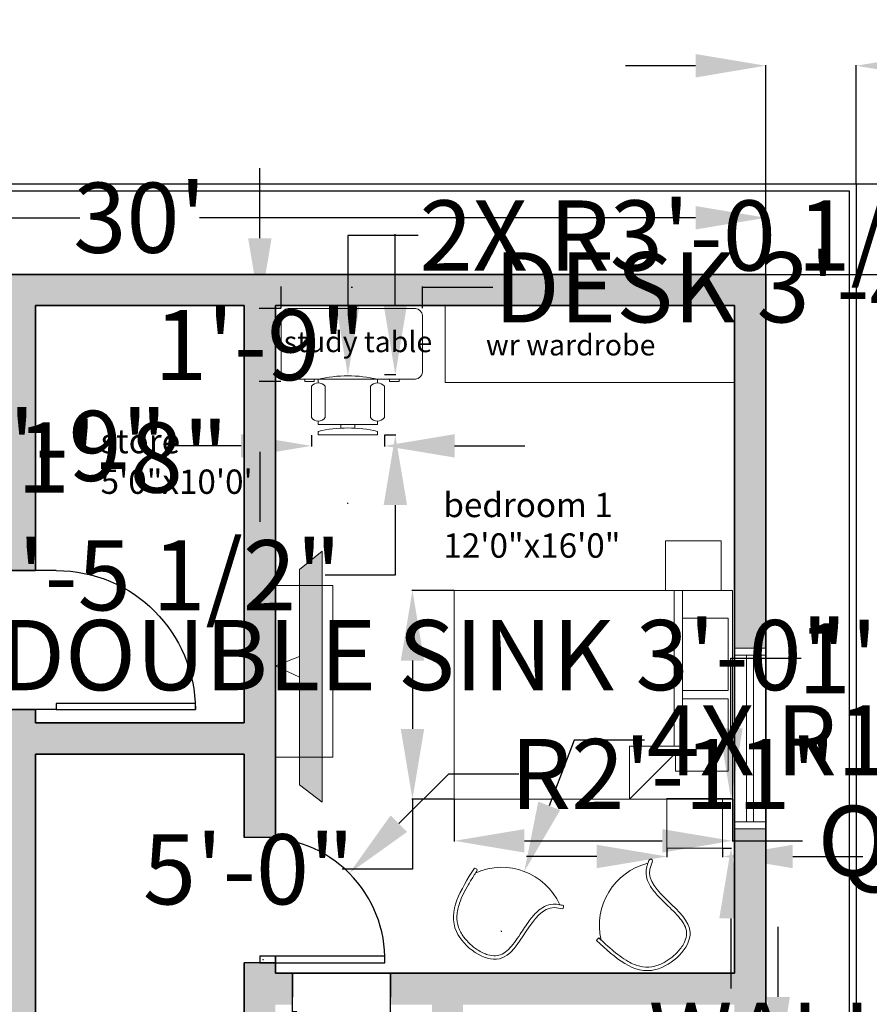
# Model space of a CAD drawing. Units: inches. Extents: x 1202 to 2101, y 998 to 1743.
# Tile 3 of 4: x 1553 to 1798, y 1460 to 1743. Entities that reach past the tile are written whole.
import ezdxf

# ---------------------------------------------------------------- set-up
doc = ezdxf.new("R2010")
doc.units = ezdxf.units.IN
doc.header["$MEASUREMENT"] = 0
for name, color, linetype, lineweight in [('A-ANNO-DIMS', 2, 'Continuous', 18), ('A-ANNO-TEXT', 7, 'Continuous', 18), ('A-AREA-IDEN', 7, 'Continuous', 18), ('A-DOOR', 3, 'Continuous', 25), ('A-FLOR-CASE', 8, 'Continuous', 18), ('A-FURN', 8, 'Continuous', 18), ('A-FURN-PATT', 250, 'Continuous', 13), ('A-GLAZ', 4, 'Continuous', 18), ('A-WALL', 7, 'Continuous', 35), ('A-WALL-PATT', 250, 'Continuous', 13), ('C-PROP', 7, 'Continuous', 30)]:
    doc.layers.add(name, color=color, linetype=linetype, lineweight=lineweight)
doc.styles.get("Standard").update_dxf_attribs({"font": 'arial.ttf'})
doc.dimstyles.get("Standard").update_dxf_attribs({"dimtxt": 20.18, "dimasz": 20.18, "dimexe": 0.18, "dimexo": 0.0625, "dimgap": 0.09, "dimtad": 0, "dimtih": 1, "dimtoh": 1, "dimdec": 0, "dimzin": 0, "dimdsep": 46, "dimlunit": 3, "dimtxsty": 'Standard', "dimcen": 0.09, "dimadec": 0, "dimazin": 0, "dimtfac": 1, "dimtdec": 0, "dimtofl": 0, "dimtmove": 0, "dimatfit": 3, "dimfxl": 1, "dimtolj": 1, "dimtzin": 0, "dimarcsym": 0})

# ---------------------------------------------------------------- blocks, each defined once
blk = doc.blocks.new('*U2')
for p, q in [((0, 0), (0, -6)), ((40, 0), (40, -6))]:
    blk.add_line(p, q)
blk.add_lwpolyline([(0, 0), (0, 40), (1.75, 40), (1.75, 0)], close=True)
blk.add_arc((0, 0), 40, 0, 90)
blk = doc.blocks.new('Bed - Queen')
for p, q in [((0, -80.00003), (0, 0)), ((0, 0), (59.99999, 0)), ((59.99999, 0), (59.99999, -80.00003)), ((7.99999, -1.2), (28.79998, -1.2)), ((7.99999, -14.4), (7.99999, -1.2)), ((28.79998, -1.2), (28.79998, -14.4)), ((31.19999, -1.2), (51.99999, -1.2)), ((31.19999, -14.4), (31.19999, -1.2)), ((51.99999, -1.2), (51.99999, -16.4)), ((0, -14.4), (44.8, -14.4)), ((44.8, -16.8), (0, -16.8)), ((59.99999, -29.6), (44.8, -14.4)), ((44.8, -14.4), (44.8, -29.6)), ((51.99999, -16.4), (46.79936, -16.4)), ((44.8, -29.6), (59.99999, -29.6)), ((59.99999, -80.00003), (0, -80.00003))]:
    blk.add_line(p, q)
blk = doc.blocks.new('Chair - Desk')
for p, q in [((-8.5, 0), (-8.5, -1)), ((-8.5, 0), (8.5, 0)), ((8.5, 0), (8.5, -1)), ((-2, -3), (-2, -1.9355)), ((2, -1.9576), (2, -3)), ((-10.5, -5), (-10.5, -14)), ((-8.5, -3), (-8.5, -4)), ((-8.5, -3), (8.5, -3)), ((-6.5, -14), (-6.5, -5)), ((6.5, -5), (6.5, -14)), ((8.5, -3), (8.5, -4)), ((10.5, -14), (10.5, -5)), ((-8.5, -15), (-8.5, -16)), ((8.5, -15), (8.5, -16))]:
    blk.add_line(p, q)
for centre, radius, start, end in [((0, 34.625), 36.625, 256.5803, 283.4197), ((-8.5, -6.5), 2.5, 36.8699, 143.1301), ((8.5, -6.5), 2.5, 36.8699, 143.1301), ((-8.5, -12.5), 2.5, 216.8699, 323.1301), ((8.5, -12.5), 2.5, 216.8699, 323.1301), ((0, 19.625), 36.625, 256.5803, 283.4197)]:
    blk.add_arc(centre, radius, start, end)
blk = doc.blocks.new('Desk - 30 x 60 in.')
for p, q in [((-26.999995, 0), (26.999995, 0)), ((-29.999995, -27), (-29.999995, -3)), ((29.999995, -3), (29.999995, -27)), ((26.999995, -30), (-26.999995, -30)), ((-20.000005, -30), (-20.000005, -31)), ((-20.000005, -31), (-16.000005, -31)), ((-16.000005, -31), (-16.000005, -30)), ((15.999995, -31), (15.999995, -30)), ((19.999995, -31), (15.999995, -31)), ((19.999995, -30), (19.999995, -31))]:
    blk.add_line(p, q)
for centre, start, end in [((-26.499995, -3.5), 98.1301, 171.8699), ((26.499995, -3.5), 8.130102, 81.8699), ((-26.499995, -26.5), 188.1301, 261.8699), ((26.499995, -26.5), 278.1301, 351.8699)]:
    blk.add_arc(centre, 3.535534, start, end)
blk = doc.blocks.new('*D9')
at = {"layer": 'A-ANNO-DIMS', "color": 0, "lineweight": -2, "transparency": 16777216}
for p, q in [((1407.98, 1669.53), (1407.98, 1685.93)), ((1428.16, 1685.75), (1570.77, 1685.75)), ((1747.8, 1685.75), (1605.18, 1685.75)), ((1767.98, 1669.53), (1767.98, 1685.93))]:
    blk.add_line(p, q, dxfattribs=at)
at = {"layer": 'A-ANNO-DIMS', "color": 0, "transparency": 16777216}
for points in [[(1428.16, 1689.11), (1428.16, 1682.38), (1407.98, 1685.75)], [(1747.8, 1689.11), (1747.8, 1682.38), (1767.98, 1685.75)]]:
    blk.add_solid(points, dxfattribs=at)
at = {"layer": 'Defpoints', "color": 0, "transparency": 16777216}
for p in [(1767.98, 1685.75), (1407.98, 1669.47), (1767.98, 1669.47)]:
    blk.add_point(p, dxfattribs=at)
at = {"layer": 'A-ANNO-DIMS', "color": 0, "transparency": 16777216, "insert": (1587.98, 1685.75), "char_height": 20.18, "attachment_point": 5}
blk.add_mtext("\\A1;30'", dxfattribs=at)
blk = doc.blocks.new('WIN-48IN-PLAN')
for p, q in [((9, 48), (0, 48)), ((3.5, 48), (3.5, 0)), ((5.5, 48), (5.5, 0)), ((9, 0), (0, 0))]:
    blk.add_line(p, q)
blk = doc.blocks.new('NIGHTSTAND-16IN')
blk.add_lwpolyline([(16, 0), (0, 0), (0, 14.24), (16, 14.24)], close=True)
blk = doc.blocks.new('*D21')
at = {"layer": 'A-ANNO-DIMS', "color": 0, "lineweight": -2, "transparency": 16777216}
for p, q in [((1771.58, 1461.65), (1771.58, 1481.83)), ((1768.04, 1441.47), (1771.76, 1441.47)), ((1768.04, 1417.47), (1771.76, 1417.47)), ((1771.58, 1397.29), (1771.58, 1377.11))]:
    blk.add_line(p, q, dxfattribs=at)
at = {"layer": 'A-ANNO-DIMS', "color": 0, "transparency": 16777216}
for points in [[(1768.21, 1461.65), (1774.94, 1461.65), (1771.58, 1441.47)], [(1768.21, 1397.29), (1774.94, 1397.29), (1771.58, 1417.47)]]:
    blk.add_solid(points, dxfattribs=at)
at = {"layer": 'Defpoints', "color": 0, "transparency": 16777216}
for p in [(1767.98, 1441.47), (1771.58, 1441.47), (1767.98, 1417.47)]:
    blk.add_point(p, dxfattribs=at)
at = {"layer": 'A-ANNO-DIMS', "color": 0, "transparency": 16777216, "insert": (1771.58, 1429.47), "char_height": 20.18, "attachment_point": 5}
blk.add_mtext('\\A1;WINDOW 2\'-0" TYP.', dxfattribs=at)
blk = doc.blocks.new('*D23')
at = {"layer": 'A-ANNO-DIMS', "color": 0, "lineweight": -2, "transparency": 16777216}
for p, q in [((1705.63, 1429.75), (1705.63, 1449.93)), ((1705.63, 1449.93), (1725.81, 1449.93)), ((1707.09, 1409.57), (1705.45, 1409.57)), ((1707.09, 1399.47), (1705.45, 1399.47)), ((1705.63, 1379.29), (1705.63, 1359.11))]:
    blk.add_line(p, q, dxfattribs=at)
at = {"layer": 'A-ANNO-DIMS', "color": 0, "transparency": 16777216}
for points in [[(1702.27, 1429.75), (1709, 1429.75), (1705.63, 1409.57)], [(1702.27, 1379.29), (1709, 1379.29), (1705.63, 1399.47)]]:
    blk.add_solid(points, dxfattribs=at)
at = {"layer": 'Defpoints', "color": 0, "transparency": 16777216}
for p in [(1705.63, 1409.57), (1707.15, 1409.57), (1707.15, 1399.47)]:
    blk.add_point(p, dxfattribs=at)
at = {"layer": 'A-ANNO-DIMS', "color": 0, "transparency": 16777216, "insert": (1896.68, 1449.93), "char_height": 20.18, "attachment_point": 5}
blk.add_mtext('\\A1;WALL FITTING 0\'-10" TYP.', dxfattribs=at)
blk = doc.blocks.new('*D27')
at = {"layer": 'A-ANNO-DIMS', "color": 0, "lineweight": -2, "transparency": 16777216}
for p, q in [((1739.58, 1504.38), (1739.58, 1501.86)), ((1755.58, 1504.38), (1755.58, 1501.86)), ((1719.4, 1502.04), (1699.22, 1502.04)), ((1775.76, 1502.04), (1795.94, 1502.04))]:
    blk.add_line(p, q, dxfattribs=at)
at = {"layer": 'A-ANNO-DIMS', "color": 0, "transparency": 16777216}
for points in [[(1719.4, 1505.41), (1719.4, 1498.68), (1739.58, 1502.04)], [(1775.76, 1505.41), (1775.76, 1498.68), (1755.58, 1502.04)]]:
    blk.add_solid(points, dxfattribs=at)
at = {"layer": 'Defpoints', "color": 0, "transparency": 16777216}
for p in [(1739.58, 1504.44), (1755.58, 1504.44), (1755.58, 1502.04)]:
    blk.add_point(p, dxfattribs=at)
at = {"layer": 'A-ANNO-DIMS', "color": 0, "transparency": 16777216, "insert": (1952.58, 1502.04), "char_height": 20.18, "attachment_point": 5}
blk.add_mtext('\\A1;NIGHTSTAND 1\'-4" TYP.', dxfattribs=at)
blk = doc.blocks.new('*D28')
at = {"layer": 'A-ANNO-DIMS', "color": 0, "lineweight": -2, "transparency": 16777216}
for p, q in [((1757.98, 1538.86), (1757.98, 1559.04)), ((1757.98, 1559.04), (1778.16, 1559.04)), ((1755.64, 1518.68), (1758.16, 1518.68)), ((1755.64, 1504.44), (1758.16, 1504.44)), ((1757.98, 1484.26), (1757.98, 1464.08))]:
    blk.add_line(p, q, dxfattribs=at)
at = {"layer": 'A-ANNO-DIMS', "color": 0, "transparency": 16777216}
for points in [[(1754.62, 1538.86), (1761.34, 1538.86), (1757.98, 1518.68)], [(1754.62, 1484.26), (1761.34, 1484.26), (1757.98, 1504.44)]]:
    blk.add_solid(points, dxfattribs=at)
at = {"layer": 'Defpoints', "color": 0, "transparency": 16777216}
for p in [(1755.58, 1518.68), (1757.98, 1518.68), (1755.58, 1504.44)]:
    blk.add_point(p, dxfattribs=at)
at = {"layer": 'A-ANNO-DIMS', "color": 0, "transparency": 16777216, "insert": (1838.8, 1559.04), "char_height": 20.18, "attachment_point": 5}
blk.add_mtext('\\A1;1\'-2" TYP.', dxfattribs=at)
blk = doc.blocks.new('*D29')
at = {"layer": 'A-ANNO-DIMS', "color": 0, "lineweight": -2, "transparency": 16777216}
for p, q in [((1678.41, 1518.49), (1678.41, 1506.37)), ((1758.41, 1518.49), (1758.41, 1506.37)), ((1698.59, 1506.55), (1738.23, 1506.55)), ((1758.41, 1506.55), (1778.59, 1506.55))]:
    blk.add_line(p, q, dxfattribs=at)
at = {"layer": 'A-ANNO-DIMS', "color": 0, "transparency": 16777216}
for points in [[(1698.59, 1509.91), (1698.59, 1503.18), (1678.41, 1506.55)], [(1738.23, 1509.91), (1738.23, 1503.18), (1758.41, 1506.55)]]:
    blk.add_solid(points, dxfattribs=at)
at = {"layer": 'Defpoints', "color": 0, "transparency": 16777216}
for p in [(1678.41, 1518.55), (1758.41, 1518.55), (1758.41, 1506.55)]:
    blk.add_point(p, dxfattribs=at)
at = {"layer": 'A-ANNO-DIMS', "color": 0, "transparency": 16777216, "insert": (1892.42, 1506.55), "char_height": 20.18, "attachment_point": 5}
blk.add_mtext('\\A1;QUEEN BED 6\'-8"', dxfattribs=at)
blk = doc.blocks.new('*D30')
at = {"layer": 'A-ANNO-DIMS', "color": 0, "lineweight": -2, "transparency": 16777216}
for p, q in [((1678.35, 1578.55), (1666.23, 1578.55)), ((1666.41, 1558.37), (1666.41, 1538.73)), ((1678.35, 1518.55), (1666.23, 1518.55)), ((1666.41, 1518.55), (1666.41, 1498.37)), ((1666.41, 1498.37), (1646.23, 1498.37))]:
    blk.add_line(p, q, dxfattribs=at)
at = {"layer": 'A-ANNO-DIMS', "color": 0, "transparency": 16777216}
for points in [[(1663.05, 1558.37), (1669.77, 1558.37), (1666.41, 1578.55)], [(1663.05, 1538.73), (1669.77, 1538.73), (1666.41, 1518.55)]]:
    blk.add_solid(points, dxfattribs=at)
at = {"layer": 'Defpoints', "color": 0, "transparency": 16777216}
for p in [(1678.41, 1578.55), (1666.41, 1518.55), (1678.41, 1518.55)]:
    blk.add_point(p, dxfattribs=at)
at = {"layer": 'A-ANNO-DIMS', "color": 0, "transparency": 16777216, "insert": (1619.32, 1498.37), "char_height": 20.18, "attachment_point": 5}
blk.add_mtext('\\A1;5\'-0"', dxfattribs=at)
blk = doc.blocks.new('*D33')
at = {"layer": 'A-ANNO-DIMS', "color": 0, "lineweight": -2, "transparency": 16777216}
for p, q in [((1467.99, 1565.29), (1467.99, 1559.78)), ((1503.99, 1565.29), (1503.99, 1559.78)), ((1447.81, 1559.96), (1427.63, 1559.96)), ((1524.17, 1559.96), (1544.35, 1559.96))]:
    blk.add_line(p, q, dxfattribs=at)
at = {"layer": 'A-ANNO-DIMS', "color": 0, "transparency": 16777216}
for points in [[(1447.81, 1563.32), (1447.81, 1556.59), (1467.99, 1559.96)], [(1524.17, 1563.32), (1524.17, 1556.59), (1503.99, 1559.96)]]:
    blk.add_solid(points, dxfattribs=at)
at = {"layer": 'Defpoints', "color": 0, "transparency": 16777216}
for p in [(1467.99, 1565.36), (1503.99, 1565.36), (1503.99, 1559.96)]:
    blk.add_point(p, dxfattribs=at)
at = {"layer": 'A-ANNO-DIMS', "color": 0, "transparency": 16777216, "insert": (1669.46, 1559.96), "char_height": 20.18, "attachment_point": 5}
blk.add_mtext('\\A1;DOUBLE SINK 3\'-0"', dxfattribs=at)
blk = doc.blocks.new('*D35')
at = {"layer": 'A-ANNO-DIMS', "color": 0, "lineweight": -2, "transparency": 16777216}
for p, q in [((1637.33, 1623.23), (1637.33, 1619.96)), ((1658.33, 1623.23), (1658.33, 1619.96)), ((1617.15, 1620.14), (1596.97, 1620.14)), ((1678.51, 1620.14), (1698.69, 1620.14))]:
    blk.add_line(p, q, dxfattribs=at)
at = {"layer": 'A-ANNO-DIMS', "color": 0, "transparency": 16777216}
for points in [[(1617.15, 1623.51), (1617.15, 1616.78), (1637.33, 1620.14)], [(1678.51, 1623.51), (1678.51, 1616.78), (1658.33, 1620.14)]]:
    blk.add_solid(points, dxfattribs=at)
at = {"layer": 'Defpoints', "color": 0, "transparency": 16777216}
for p in [(1637.33, 1623.29), (1658.33, 1623.29), (1637.33, 1620.14)]:
    blk.add_point(p, dxfattribs=at)
at = {"layer": 'A-ANNO-DIMS', "color": 0, "transparency": 16777216, "insert": (1522.41, 1620.14), "char_height": 20.18, "attachment_point": 5}
blk.add_mtext('\\A1;CHAIR 1\'-9"', dxfattribs=at)
blk = doc.blocks.new('*D36')
at = {"layer": 'A-ANNO-DIMS', "color": 0, "lineweight": -2, "transparency": 16777216}
for p, q in [((1661.48, 1660.81), (1661.48, 1680.99)), ((1658.4, 1640.63), (1661.66, 1640.63)), ((1658.4, 1623.29), (1661.66, 1623.29)), ((1661.48, 1603.11), (1661.48, 1582.93)), ((1661.48, 1582.93), (1641.3, 1582.93))]:
    blk.add_line(p, q, dxfattribs=at)
at = {"layer": 'A-ANNO-DIMS', "color": 0, "transparency": 16777216}
for points in [[(1658.12, 1660.81), (1664.85, 1660.81), (1661.48, 1640.63)], [(1658.12, 1603.11), (1664.85, 1603.11), (1661.48, 1623.29)]]:
    blk.add_solid(points, dxfattribs=at)
at = {"layer": 'Defpoints', "color": 0, "transparency": 16777216}
for p in [(1658.33, 1640.63), (1658.33, 1623.29), (1661.48, 1623.29)]:
    blk.add_point(p, dxfattribs=at)
at = {"layer": 'A-ANNO-DIMS', "color": 0, "transparency": 16777216, "insert": (1591.83, 1582.93), "char_height": 20.18, "attachment_point": 5}
blk.add_mtext('\\A1;1\'-5 1/2"', dxfattribs=at)
blk = doc.blocks.new('*D37')
at = {"layer": 'A-ANNO-DIMS', "color": 0, "lineweight": -2, "transparency": 16777216}
for p, q in [((1628.63, 1659.71), (1628.63, 1665.93)), ((1648.81, 1665.75), (1649.15, 1665.75)), ((1669.33, 1659.71), (1669.33, 1665.93)), ((1669.33, 1665.75), (1689.51, 1665.75))]:
    blk.add_line(p, q, dxfattribs=at)
at = {"layer": 'A-ANNO-DIMS', "color": 0, "transparency": 16777216}
for points in [[(1648.81, 1669.11), (1648.81, 1662.39), (1628.63, 1665.75)], [(1649.15, 1669.11), (1649.15, 1662.39), (1669.33, 1665.75)]]:
    blk.add_solid(points, dxfattribs=at)
at = {"layer": 'Defpoints', "color": 0, "transparency": 16777216}
for p in [(1669.33, 1665.75), (1628.63, 1659.65), (1669.33, 1659.65)]:
    blk.add_point(p, dxfattribs=at)
at = {"layer": 'A-ANNO-DIMS', "color": 0, "transparency": 16777216, "insert": (1781.74, 1665.75), "char_height": 20.18, "attachment_point": 5}
blk.add_mtext('\\A1;DESK 3\'-4 1/2"', dxfattribs=at)
blk = doc.blocks.new('*D38')
at = {"layer": 'A-ANNO-DIMS', "color": 0, "lineweight": -2, "transparency": 16777216}
for p, q in [((1622.53, 1679.83), (1622.53, 1700.01)), ((1628.57, 1659.65), (1622.35, 1659.65)), ((1628.57, 1638.62), (1622.35, 1638.62)), ((1622.53, 1618.44), (1622.53, 1598.26))]:
    blk.add_line(p, q, dxfattribs=at)
at = {"layer": 'A-ANNO-DIMS', "color": 0, "transparency": 16777216}
for points in [[(1619.16, 1679.83), (1625.89, 1679.83), (1622.53, 1659.65)], [(1619.16, 1618.44), (1625.89, 1618.44), (1622.53, 1638.62)]]:
    blk.add_solid(points, dxfattribs=at)
at = {"layer": 'Defpoints', "color": 0, "transparency": 16777216}
for p in [(1622.53, 1659.65), (1628.63, 1659.65), (1628.63, 1638.62)]:
    blk.add_point(p, dxfattribs=at)
at = {"layer": 'A-ANNO-DIMS', "color": 0, "transparency": 16777216, "insert": (1622.53, 1649.13), "char_height": 20.18, "attachment_point": 5}
blk.add_mtext('\\A1;1\'-9"', dxfattribs=at)
blk = doc.blocks.new('*D42')
at = {"layer": 'A-ANNO-DIMS', "color": 0, "lineweight": -2, "transparency": 16777216}
for p, q in [((1768.04, 1669.47), (1853.16, 1669.47)), ((1852.98, 1649.29), (1852.98, 1471.37)), ((1852.98, 1272.65), (1852.98, 1450.57)), ((1618.04, 1252.47), (1853.16, 1252.47))]:
    blk.add_line(p, q, dxfattribs=at)
at = {"layer": 'A-ANNO-DIMS', "color": 0, "transparency": 16777216}
for points in [[(1849.61, 1649.29), (1856.34, 1649.29), (1852.98, 1669.47)], [(1849.61, 1272.65), (1856.34, 1272.65), (1852.98, 1252.47)]]:
    blk.add_solid(points, dxfattribs=at)
at = {"layer": 'Defpoints', "color": 0, "transparency": 16777216}
for p in [(1767.98, 1669.47), (1852.98, 1669.47), (1617.98, 1252.47)]:
    blk.add_point(p, dxfattribs=at)
at = {"layer": 'A-ANNO-DIMS', "color": 0, "transparency": 16777216, "insert": (1852.98, 1460.97), "char_height": 20.18, "attachment_point": 5}
blk.add_mtext('\\A1;34\'-9"', dxfattribs=at)
blk = doc.blocks.new('*D43')
at = {"layer": 'A-ANNO-DIMS', "color": 0, "lineweight": -2, "transparency": 16777216}
for p, q in [((1852.98, 1715.65), (1852.98, 1735.83)), ((1794.04, 1695.47), (1853.16, 1695.47)), ((1768.04, 1669.47), (1853.16, 1669.47)), ((1852.98, 1649.29), (1852.98, 1629.11))]:
    blk.add_line(p, q, dxfattribs=at)
at = {"layer": 'A-ANNO-DIMS', "color": 0, "transparency": 16777216}
for points in [[(1849.61, 1715.65), (1856.34, 1715.65), (1852.98, 1695.47)], [(1849.61, 1649.29), (1856.34, 1649.29), (1852.98, 1669.47)]]:
    blk.add_solid(points, dxfattribs=at)
at = {"layer": 'Defpoints', "color": 0, "transparency": 16777216}
for p in [(1793.98, 1695.47), (1852.98, 1695.47), (1767.98, 1669.47)]:
    blk.add_point(p, dxfattribs=at)
at = {"layer": 'A-ANNO-DIMS', "color": 0, "transparency": 16777216, "insert": (1852.98, 1682.47), "char_height": 20.18, "attachment_point": 5}
blk.add_mtext('\\A1;2\'-2"', dxfattribs=at)
blk = doc.blocks.new('*D45')
at = {"layer": 'A-ANNO-DIMS', "color": 0, "lineweight": -2, "transparency": 16777216}
for p, q in [((1747.8, 1729.47), (1727.62, 1729.47)), ((1767.98, 1669.53), (1767.98, 1729.65)), ((1793.98, 1695.53), (1793.98, 1729.65)), ((1814.16, 1729.47), (1834.34, 1729.47))]:
    blk.add_line(p, q, dxfattribs=at)
at = {"layer": 'A-ANNO-DIMS', "color": 0, "transparency": 16777216}
for points in [[(1747.8, 1732.83), (1747.8, 1726.1), (1767.98, 1729.47)], [(1814.16, 1732.83), (1814.16, 1726.1), (1793.98, 1729.47)]]:
    blk.add_solid(points, dxfattribs=at)
at = {"layer": 'Defpoints', "color": 0, "transparency": 16777216}
for p in [(1793.98, 1729.47), (1793.98, 1695.47), (1767.98, 1669.47)]:
    blk.add_point(p, dxfattribs=at)
at = {"layer": 'A-ANNO-DIMS', "color": 0, "transparency": 16777216, "insert": (1861.42, 1729.47), "char_height": 20.18, "attachment_point": 5}
blk.add_mtext('\\A1;2\'-2"', dxfattribs=at)
blk = doc.blocks.new('*D48')
at = {"layer": 'A-ANNO-DIMS', "color": 0, "lineweight": -2, "transparency": 16777216}
for p, q in [((1668.02, 1680.65), (1647.84, 1680.65)), ((1647.84, 1680.65), (1647.84, 1660.47)), ((1647.74, 1603.67), (1647.92, 1603.67)), ((1647.83, 1603.58), (1647.83, 1603.76))]:
    blk.add_line(p, q, dxfattribs=at)
at = {"layer": 'A-ANNO-DIMS', "color": 0, "transparency": 16777216}
blk.add_solid([(1644.47, 1660.47), (1651.2, 1660.47), (1647.84, 1640.29)], dxfattribs=at)
at = {"layer": 'Defpoints', "color": 0, "transparency": 16777216}
for p in [(1647.84, 1640.29), (1647.83, 1603.67)]:
    blk.add_point(p, dxfattribs=at)
at = {"layer": 'A-ANNO-DIMS', "color": 0, "transparency": 16777216, "insert": (1749.95, 1680.65), "char_height": 20.18, "attachment_point": 5}
blk.add_mtext('\\A1;2X R3\'-0 1/2"', dxfattribs=at)
blk = doc.blocks.new('*D49')
at = {"layer": 'A-ANNO-DIMS', "color": 0, "lineweight": -2, "transparency": 16777216}
for p, q in [((1676.78, 1525.76), (1662.51, 1511.49)), ((1696.96, 1525.76), (1676.78, 1525.76)), ((1623.48, 1472.38), (1623.48, 1472.56)), ((1623.39, 1472.47), (1623.57, 1472.47))]:
    blk.add_line(p, q, dxfattribs=at)
at = {"layer": 'A-ANNO-DIMS', "color": 0, "transparency": 16777216}
blk.add_solid([(1660.13, 1513.87), (1664.88, 1509.12), (1648.24, 1497.22)], dxfattribs=at)
at = {"layer": 'Defpoints', "color": 0, "transparency": 16777216}
for p in [(1648.24, 1497.22), (1623.48, 1472.47)]:
    blk.add_point(p, dxfattribs=at)
at = {"layer": 'A-ANNO-DIMS', "color": 0, "transparency": 16777216, "insert": (1741.36, 1525.76), "char_height": 20.18, "attachment_point": 5}
blk.add_mtext('\\A1;R2\'-11"', dxfattribs=at)
blk = doc.blocks.new('*D50')
at = {"layer": 'A-ANNO-DIMS', "color": 0, "lineweight": -2, "transparency": 16777216}
for p, q in [((1712.91, 1535.47), (1705.73, 1516.61)), ((1733.09, 1535.47), (1712.91, 1535.47)), ((1691.93, 1480.57), (1692.11, 1480.57)), ((1692.02, 1480.48), (1692.02, 1480.66))]:
    blk.add_line(p, q, dxfattribs=at)
at = {"layer": 'A-ANNO-DIMS', "color": 0, "transparency": 16777216}
blk.add_solid([(1702.59, 1517.81), (1708.88, 1515.41), (1698.56, 1497.75)], dxfattribs=at)
at = {"layer": 'Defpoints', "color": 0, "transparency": 16777216}
for p in [(1698.56, 1497.75), (1692.02, 1480.57)]:
    blk.add_point(p, dxfattribs=at)
at = {"layer": 'A-ANNO-DIMS', "color": 0, "transparency": 16777216, "insert": (1815.26, 1535.47), "char_height": 20.18, "attachment_point": 5}
blk.add_mtext('\\A1;4X R1\'-6 1/2"', dxfattribs=at)
blk = doc.blocks.new('*D51')
at = {"layer": 'A-ANNO-DIMS', "color": 0, "lineweight": -2, "transparency": 16777216}
for p, q in [((1440.93, 1616.8), (1441.11, 1616.8)), ((1441.02, 1616.71), (1441.02, 1616.89)), ((1491.46, 1616.8), (1471.28, 1616.8))]:
    blk.add_line(p, q, dxfattribs=at)
at = {"layer": 'A-ANNO-DIMS', "color": 0, "transparency": 16777216}
blk.add_solid([(1471.28, 1620.16), (1471.28, 1613.43), (1451.1, 1616.8)], dxfattribs=at)
at = {"layer": 'Defpoints', "color": 0, "transparency": 16777216}
for p in [(1430.93, 1616.8), (1451.1, 1616.8)]:
    blk.add_point(p, dxfattribs=at)
at = {"layer": 'A-ANNO-DIMS', "color": 0, "transparency": 16777216, "insert": (1550.67, 1616.8), "char_height": 20.18, "attachment_point": 5}
blk.add_mtext('\\A1;2X ∅1\'-8"', dxfattribs=at)

msp = doc.modelspace()

# ---------------------------------------------------------------- hatches: boundary and pattern name
at = {"layer": 'A-FURN-PATT'}
h = msp.add_hatch(color=256, dxfattribs=at)
h.dxf.hatch_style = 1
h.paths.add_polyline_path([(1640.43, 1579.95), (1633.97, 1579.95), (1633.97, 1530.64), (1640.43, 1530.64)])
h.paths.add_polyline_path([(1640.43, 1589.86), (1633.97, 1584.6), (1633.97, 1579.95), (1640.43, 1579.95)])
h.paths.add_polyline_path([(1640.43, 1530.64), (1633.97, 1530.64), (1633.97, 1522.63), (1640.43, 1517.71)])
at = {"layer": 'A-WALL-PATT'}
h = msp.add_hatch(color=256, dxfattribs=at)
h.dxf.hatch_style = 1
h.paths.add_polyline_path([(1767.98, 1669.47), (1407.98, 1669.47), (1407.98, 1552.97), (1416.98, 1552.97), (1416.98, 1591.47), (1527.46, 1591.47), (1527.46, 1600.47), (1416.98, 1600.47), (1416.98, 1660.47), (1548.98, 1660.47), (1548.98, 1600.47), (1544.75, 1600.47), (1544.75, 1591.47), (1548.98, 1591.47), (1548.98, 1584.29), (1557.98, 1584.29), (1557.98, 1660.47), (1617.98, 1660.47), (1617.98, 1540.47), (1557.98, 1540.47), (1557.98, 1544.29), (1548.98, 1544.29), (1548.98, 1462.47), (1416.98, 1462.47), (1416.98, 1500.97), (1407.98, 1500.97), (1407.98, 1424.63), (1416.98, 1424.63), (1416.98, 1431.74), (1416.98, 1453.47), (1557.98, 1453.47), (1557.98, 1531.47), (1617.98, 1531.47), (1617.98, 1507.47), (1622.48, 1507.47, -0.014283), (1624.48, 1507.47), (1626.98, 1507.47), (1626.98, 1660.47), (1758.98, 1660.47), (1758.98, 1638.32), (1758.98, 1561.97), (1767.98, 1561.97)])
h.paths.add_polyline_path([(1416.98, 1372.63), (1407.98, 1372.63), (1407.98, 1318.84), (1416.98, 1318.84)])
h.paths.add_polyline_path([(1626.98, 1390.47), (1758.98, 1390.47), (1758.98, 1369.1), (1758.98, 1344.47), (1767.98, 1344.47), (1767.98, 1415.47), (1758.98, 1415.47), (1758.98, 1399.47), (1680.98, 1399.47), (1680.98, 1425.58), (1671.98, 1425.58), (1671.98, 1399.47), (1626.98, 1399.47), (1626.98, 1459.47), (1631.88, 1459.47), (1631.88, 1461.58), (1631.88, 1468.47), (1626.98, 1468.47), (1626.98, 1471.47), (1622.48, 1471.47), (1617.98, 1471.47), (1617.98, 1261.47), (1614.74, 1261.47), (1614.74, 1258.47), (1614.74, 1252.47), (1617.98, 1252.47), (1617.98, 1144.47), (1758.98, 1144.47), (1758.98, 1125.47), (1767.98, 1125.47), (1767.98, 1169.47), (1758.98, 1169.47), (1758.98, 1153.47), (1680.98, 1153.47), (1680.98, 1179.68, -0.04329), (1676.17, 1179.26), (1671.98, 1179.26), (1671.98, 1153.47), (1626.98, 1153.47), (1626.98, 1213.47), (1631.88, 1213.47), (1631.88, 1218.24), (1631.88, 1222.47), (1626.98, 1222.47)])
h.paths.add_polyline_path([(1767.98, 1509.97), (1758.98, 1509.97), (1758.98, 1468.47), (1660.05, 1468.47), (1660.05, 1461.58), (1660.05, 1459.47), (1671.98, 1459.47), (1671.98, 1453.51), (1680.98, 1453.51), (1680.98, 1459.47), (1758.98, 1459.47), (1758.98, 1443.47), (1767.98, 1443.47)], flags=17)
h.paths.add_polyline_path([(1767.98, 1268.47), (1758.98, 1268.47), (1758.98, 1263.28), (1758.98, 1222.47), (1660.05, 1222.47), (1660.05, 1218.24, -0.04262), (1659.64, 1213.47), (1671.98, 1213.47), (1671.98, 1207.19), (1676.17, 1207.19), (1680.98, 1207.19), (1680.98, 1213.47), (1758.98, 1213.47), (1758.98, 1197.47), (1767.98, 1197.47)], flags=17)
h.paths.add_polyline_path([(1767.98, 1073.47), (1758.98, 1073.47), (1758.98, 1054.47), (1767.98, 1054.47)])

# ---------------------------------------------------------------- linework, layer by layer
at = {"layer": 'A-DOOR'}
for p, q in [((1626.98, 1507.47), (1617.98, 1507.47)), ((1622.48, 1473.47), (1658.48, 1473.47)), ((1622.48, 1473.47), (1622.48, 1471.47)), ((1626.98, 1471.47), (1617.98, 1471.47)), ((1622.48, 1471.47), (1658.48, 1471.47))]:
    msp.add_line(p, q, dxfattribs=at)
msp.add_arc((1623.48, 1472.47), 35.01, 358.3634, 91.6366, dxfattribs=at)
at = {"layer": 'A-FLOR-CASE'}
for p, q in [((1675.77, 1638.32), (1675.77, 1660.47)), ((1758.98, 1660.47), (1758.98, 1638.32)), ((1758.98, 1638.32), (1675.77, 1638.32))]:
    msp.add_line(p, q, dxfattribs=at)
at = {"layer": 'A-FURN'}
for p, q in [((1633.97, 1584.6), (1640.43, 1589.86)), ((1640.43, 1589.86), (1640.43, 1517.71)), ((1633.97, 1522.63), (1633.97, 1584.6)), ((1626.98, 1556.86), (1633.97, 1559.55)), ((1626.98, 1556.86), (1633.97, 1553.62)), ((1640.43, 1517.71), (1633.97, 1522.63))]:
    msp.add_line(p, q, dxfattribs=at)
msp.add_lwpolyline([(1626.98, 1579.95), (1643.51, 1579.95), (1643.51, 1530.64), (1626.98, 1530.64)], close=True, dxfattribs=at)
for centre, radius, start, end in [((1734.9, 1500.74), 0.54, 0, 135.4284), ((1684.3, 1497.87), 0.79, 18.3905, 96.9055), ((1692.02, 1480.57), 18.38, 24.4629, 113.8625), ((1738.53, 1482.26), 18.38, 103.9163, 193.3158), ((1708.9, 1487.66), 0.98, 317.6007, 18.921), ((1721.08, 1476.94), 1.99, 122.5719, 151.6308)]:
    msp.add_arc(centre, radius, start, end, dxfattribs=at)
for points, knots in [([(1720.01, 1478.62), (1720.41, 1478.25), (1720.81, 1477.87), (1722.02, 1476.77), (1722.82, 1476.04), (1725.21, 1473.98), (1726.81, 1472.76), (1729.54, 1471.22), (1730.67, 1470.74), (1732.95, 1470.2), (1734.09, 1470.13), (1735.74, 1470.39), (1736.22, 1470.51), (1737.21, 1470.83), (1737.71, 1471.04), (1739.78, 1472.04), (1741.32, 1473.18), (1743.36, 1475.33), (1744.03, 1476.25), (1744.86, 1477.89), (1745.1, 1478.6), (1745.29, 1479.96), (1745.24, 1480.58), (1744.86, 1481.88), (1744.53, 1482.54), (1743.63, 1483.9), (1743.07, 1484.59), (1741.8, 1485.97), (1741.09, 1486.67), (1739.27, 1488.43), (1738.12, 1489.51), (1736.23, 1491.53), (1735.46, 1492.47), (1734.4, 1494.18), (1734.04, 1494.94), (1733.6, 1496.54), (1733.51, 1497.39), (1733.66, 1498.57), (1733.73, 1498.88), (1733.9, 1499.49), (1734, 1499.78), (1734.24, 1500.43), (1734.38, 1500.78), (1734.52, 1501.12)], [0, 0, 0, 0, 1.423574, 1.423574, 4.270721, 4.270721, 9.965016, 9.965016, 14.007628, 14.007628, 18.050241, 18.050241, 19.670932, 19.670932, 21.291623, 21.291623, 26.38725, 26.38725, 29.733224, 29.733224, 32.363164, 32.363164, 34.993104, 34.993104, 37.623043, 37.623043, 40.252983, 40.252983, 42.882923, 42.882923, 46.855545, 46.855545, 50.084133, 50.084133, 52.435754, 52.435754, 54.787375, 54.787375, 55.637603, 55.637603, 56.487831, 56.487831, 57.549481, 57.549481, 57.549481, 57.549481]), ([(1684.21, 1498.66), (1680.3, 1492.49), (1673.37, 1481.55), (1695.96, 1465.19), (1700.7, 1488.85), (1708.8, 1487.16), (1709.62, 1486.99)], [0, 0, 0, 0, 18.893928, 33.537423, 55.121312, 57.549481, 57.549481, 57.549481, 57.549481]), ([(1685.05, 1498.12), (1684.76, 1497.66), (1684.47, 1497.19), (1683.6, 1495.81), (1683.03, 1494.89), (1681.44, 1492.16), (1680.53, 1490.36), (1679.52, 1487.39), (1679.26, 1486.19), (1679.14, 1483.86), (1679.28, 1482.73), (1679.84, 1481.15), (1680.05, 1480.69), (1680.54, 1479.78), (1680.84, 1479.33), (1682.2, 1477.48), (1683.6, 1476.17), (1686.09, 1474.56), (1687.12, 1474.07), (1688.88, 1473.55), (1689.63, 1473.45), (1690.99, 1473.51), (1691.6, 1473.67), (1692.8, 1474.29), (1693.4, 1474.73), (1694.56, 1475.86), (1695.14, 1476.54), (1696.27, 1478.05), (1696.82, 1478.87), (1698.22, 1480.98), (1699.07, 1482.31), (1700.72, 1484.53), (1701.49, 1485.47), (1702.99, 1486.82), (1703.67, 1487.31), (1705.16, 1488.04), (1705.98, 1488.28), (1707.16, 1488.35), (1707.48, 1488.34), (1708.11, 1488.28), (1708.42, 1488.24), (1709.1, 1488.12), (1709.47, 1488.05), (1709.82, 1487.97)], [0, 0, 0, 0, 1.423574, 1.423574, 4.270721, 4.270721, 9.965016, 9.965016, 14.007628, 14.007628, 18.050241, 18.050241, 19.670932, 19.670932, 21.291623, 21.291623, 26.38725, 26.38725, 29.733224, 29.733224, 32.363164, 32.363164, 34.993104, 34.993104, 37.623043, 37.623043, 40.252983, 40.252983, 42.882923, 42.882923, 46.855545, 46.855545, 50.084133, 50.084133, 52.435754, 52.435754, 54.787375, 54.787375, 55.637603, 55.637603, 56.487831, 56.487831, 57.549481, 57.549481, 57.549481, 57.549481]), ([(1719.33, 1477.89), (1724.67, 1472.92), (1734.16, 1464.11), (1754.38, 1483.32), (1731.99, 1492.31), (1735.13, 1499.96), (1735.44, 1500.74)], [0, 0, 0, 0, 18.893928, 33.537423, 55.121312, 57.549481, 57.549481, 57.549481, 57.549481])]:
    msp.add_open_spline(points, degree=3, knots=knots, dxfattribs=at)
at = {"layer": 'A-GLAZ'}
for p, q in [((1758.98, 1561.97), (1767.98, 1561.97)), ((1758.98, 1509.97), (1767.98, 1509.97))]:
    msp.add_line(p, q, dxfattribs=at)
at = {"layer": 'A-WALL'}
for p, q in [((1407.98, 1669.47), (1767.98, 1669.47)), ((1767.98, 1669.47), (1767.98, 1054.47)), ((1557.98, 1660.47), (1617.98, 1660.47)), ((1557.98, 1584.29), (1557.98, 1660.47)), ((1617.98, 1540.47), (1617.98, 1660.47)), ((1626.98, 1660.47), (1758.98, 1660.47)), ((1626.98, 1507.31), (1626.98, 1660.47)), ((1626.98, 1507.31), (1626.98, 1660.47)), ((1758.98, 1660.47), (1758.98, 1540.47)), ((1557.98, 1584.29), (1548.98, 1584.29)), ((1557.98, 1544.29), (1548.98, 1544.29)), ((1557.98, 1540.47), (1557.98, 1544.29)), ((1557.98, 1540.47), (1617.98, 1540.47)), ((1758.98, 1540.47), (1758.98, 1531.47)), ((1557.98, 1453.47), (1557.98, 1531.47)), ((1557.98, 1531.47), (1617.98, 1531.47)), ((1617.98, 1507.47), (1617.98, 1531.47)), ((1758.98, 1531.47), (1758.98, 1468.47)), ((1626.98, 1468.47), (1626.98, 1473.47)), ((1626.98, 1468.47), (1626.98, 1473.47)), ((1617.98, 1261.47), (1617.98, 1471.47)), ((1626.98, 1468.47), (1630.13, 1468.47)), ((1626.98, 1468.47), (1758.98, 1468.47)), ((1631.88, 1461.58), (1631.88, 1468.47)), ((1660.05, 1461.58), (1660.05, 1468.47))]:
    msp.add_line(p, q, dxfattribs=at)
at = {"layer": 'C-PROP'}
for p, q in [((1381.98, 1695.47), (1793.98, 1695.47)), ((1383.98, 1693.47), (1791.98, 1693.47)), ((1791.98, 1693.47), (1791.98, 1054.47)), ((1793.98, 1695.47), (1793.98, 1045.47))]:
    msp.add_line(p, q, dxfattribs=at)

# ---------------------------------------------------------------- block references
at = {"layer": 'A-DOOR', "xscale": -1, "rotation": 270}
msp.add_blockref('*U2', (1563.98, 1544.29), dxfattribs=at)
at = {"layer": 'A-DOOR', "xscale": -0.7041064892560387, "yscale": 0.7041064892560387, "zscale": 0.7041064892560387, "rotation": 180}
msp.add_blockref('*U2', (1631.88, 1457.35), dxfattribs=at)
at = {"layer": 'A-FURN', "xscale": 0.678389605659127, "yscale": 0.678389605659127, "zscale": 0.678389605659127}
msp.add_blockref('Desk - 30 x 60 in.', (1648.98, 1659.65), dxfattribs=at)
at = {"layer": 'A-FURN'}
for name, p, rotation in [('Chair - Desk', (1647.83, 1623.29), 180), ('Bed - Queen', (1758.41, 1578.55), 270)]:
    msp.add_blockref(name, p, dxfattribs=dict(at, rotation=rotation))
for p in [(1739.18, 1578.55), (1739.58, 1504.44)]:
    msp.add_blockref('NIGHTSTAND-16IN', p, dxfattribs=at)
at = {"layer": 'A-GLAZ'}
msp.add_blockref('WIN-48IN-PLAN', (1758.98, 1511.97), dxfattribs=at)

# ---------------------------------------------------------------- texts
at = {"layer": 'A-ANNO-TEXT', "char_height": 6, "attachment_point": 1}
for s, insert in [('study table', (1629.41, 1653.09)), ('wr wardrobe', (1687.53, 1652.15))]:
    msp.add_mtext_dynamic_manual_height_columns(s, width=58.9988, gutter_width=1, heights=[0], dxfattribs=dict(at, insert=insert))
at = {"layer": 'A-AREA-IDEN', "char_height": 7, "attachment_point": 1}
for s, width, insert in [('store\\P5\'0"x10\'0\'', 28.6147, (1576.74, 1625.01)), ('bedroom 1\\P12\'0"x16\'0"', 54.5484, (1675.3, 1606.65))]:
    msp.add_mtext_dynamic_manual_height_columns(s, width=width, gutter_width=1, heights=[0], dxfattribs=dict(at, insert=insert))

# ---------------------------------------------------------------- dimensions: what is measured, and where the dimension line sits
at = {"layer": 'A-ANNO-DIMS'}
for base, p1, p2, override, picture, middle in [((1793.98, 1729.47), (1767.98, 1669.47), (1793.98, 1695.47), {"dimdec": 1, "dimlfac": 1, "dimrnd": 0, "dimzin": 1, "dimdsep": 46, "dimlunit": 4, "dimfrac": 2}, '*D45', (1861.42, 1729.47)), ((1767.98, 1685.75), (1407.98, 1669.47), (1767.98, 1669.47), {"dimclrd": 0, "dimclre": 0, "dimclrt": 0}, '*D9', (1587.98, 1685.75))]:
    dim = msp.add_linear_dim(base=base, p1=p1, p2=p2, dimstyle='Standard', override=override, dxfattribs=at)
    dim.commit()
    dim.dimension.update_dxf_attribs({"geometry": picture, "text_midpoint": middle})
for base, p1, p2, angle, picture, middle in [((1852.98, 1695.47), (1767.98, 1669.47), (1793.98, 1695.47), 90, '*D43', (1852.98, 1682.47)), ((1622.53, 1659.65), (1628.63, 1638.62), (1628.63, 1659.65), 90, '*D38', (1622.53, 1649.13)), ((1661.48, 1623.29), (1658.33, 1640.63), (1658.33, 1623.29), 270, '*D36', (1591.83, 1582.93)), ((1852.98, 1669.47), (1617.98, 1252.47), (1767.98, 1669.47), 90, '*D42', (1852.98, 1460.97)), ((1666.41, 1518.55), (1678.41, 1578.55), (1678.41, 1518.55), 270, '*D30', (1619.32, 1498.37))]:
    dim = msp.add_linear_dim(base=base, p1=p1, p2=p2, angle=angle, dimstyle='Standard', override={"dimdec": 1, "dimlfac": 1, "dimrnd": 0, "dimzin": 1, "dimdsep": 46, "dimlunit": 4, "dimfrac": 2}, dxfattribs=at)
    dim.commit()
    dim.dimension.update_dxf_attribs({"geometry": picture, "text_midpoint": middle})
for center, mpoint, text, picture, middle in [((1647.83, 1603.67), (1647.84, 1640.29), '2X <>', '*D48', (1749.95, 1680.65)), ((1692.02, 1480.57), (1698.56, 1497.75), '4X <>', '*D50', (1815.26, 1535.47))]:
    dim = msp.add_radius_dim(center=center, mpoint=mpoint, text=text, dimstyle='Standard', override={"dimdec": 1, "dimlfac": 1, "dimrnd": 0, "dimzin": 1, "dimdsep": 46, "dimlunit": 4, "dimfrac": 2}, dxfattribs=at)
    dim.commit()
    dim.dimension.update_dxf_attribs({"geometry": picture, "text_midpoint": middle})
for base, p1, p2, text, picture, middle in [((1669.33, 1665.75), (1628.63, 1659.65), (1669.33, 1659.65), 'DESK <>', '*D37', (1781.74, 1665.75)), ((1503.99, 1559.96), (1467.99, 1565.36), (1503.99, 1565.36), 'DOUBLE SINK <>', '*D33', (1669.46, 1559.96)), ((1758.41, 1506.55), (1678.41, 1518.55), (1758.41, 1518.55), 'QUEEN BED <>', '*D29', (1892.42, 1506.55)), ((1755.58, 1502.04), (1739.58, 1504.44), (1755.58, 1504.44), 'NIGHTSTAND <> TYP.', '*D27', (1952.58, 1502.04))]:
    dim = msp.add_linear_dim(base=base, p1=p1, p2=p2, text=text, dimstyle='Standard', override={"dimdec": 1, "dimlfac": 1, "dimrnd": 0, "dimzin": 1, "dimdsep": 46, "dimlunit": 4, "dimfrac": 2}, dxfattribs=at)
    dim.commit()
    dim.dimension.update_dxf_attribs({"geometry": picture, "text_midpoint": middle})
for base, p1, p2, angle, text, picture, middle in [((1637.33, 1620.14), (1658.33, 1623.29), (1637.33, 1623.29), 180, 'CHAIR <>', '*D35', (1522.41, 1620.14)), ((1757.98, 1518.68), (1755.58, 1504.44), (1755.58, 1518.68), 90, '<> TYP.', '*D28', (1838.8, 1559.04)), ((1705.63, 1409.57), (1707.15, 1399.47), (1707.15, 1409.57), 90, 'WALL FITTING <> TYP.', '*D23', (1896.68, 1449.93)), ((1771.58, 1441.47), (1767.98, 1417.47), (1767.98, 1441.47), 90, 'WINDOW <> TYP.', '*D21', (1771.58, 1429.47))]:
    dim = msp.add_linear_dim(base=base, p1=p1, p2=p2, angle=angle, text=text, dimstyle='Standard', override={"dimdec": 1, "dimlfac": 1, "dimrnd": 0, "dimzin": 1, "dimdsep": 46, "dimlunit": 4, "dimfrac": 2}, dxfattribs=at)
    dim.commit()
    dim.dimension.update_dxf_attribs({"geometry": picture, "text_midpoint": middle})
dim = msp.add_diameter_dim_2p(p1=(1430.93, 1616.8), p2=(1451.1, 1616.8), text='2X <>', dimstyle='Standard', override={"dimdec": 1, "dimlfac": 1, "dimrnd": 0, "dimzin": 1, "dimdsep": 46, "dimlunit": 4, "dimfrac": 2}, dxfattribs=at)
dim.commit()
dim.dimension.update_dxf_attribs({"geometry": '*D51', "text_midpoint": (1491.46, 1616.8)})
dim = msp.add_radius_dim(center=(1623.48, 1472.47), mpoint=(1648.24, 1497.22), dimstyle='Standard', override={"dimdec": 1, "dimlfac": 1, "dimrnd": 0, "dimzin": 1, "dimdsep": 46, "dimlunit": 4, "dimfrac": 2}, dxfattribs=at)
dim.commit()
dim.dimension.update_dxf_attribs({"geometry": '*D49', "text_midpoint": (1741.36, 1525.76)})

doc.saveas('drawing.dxf')
